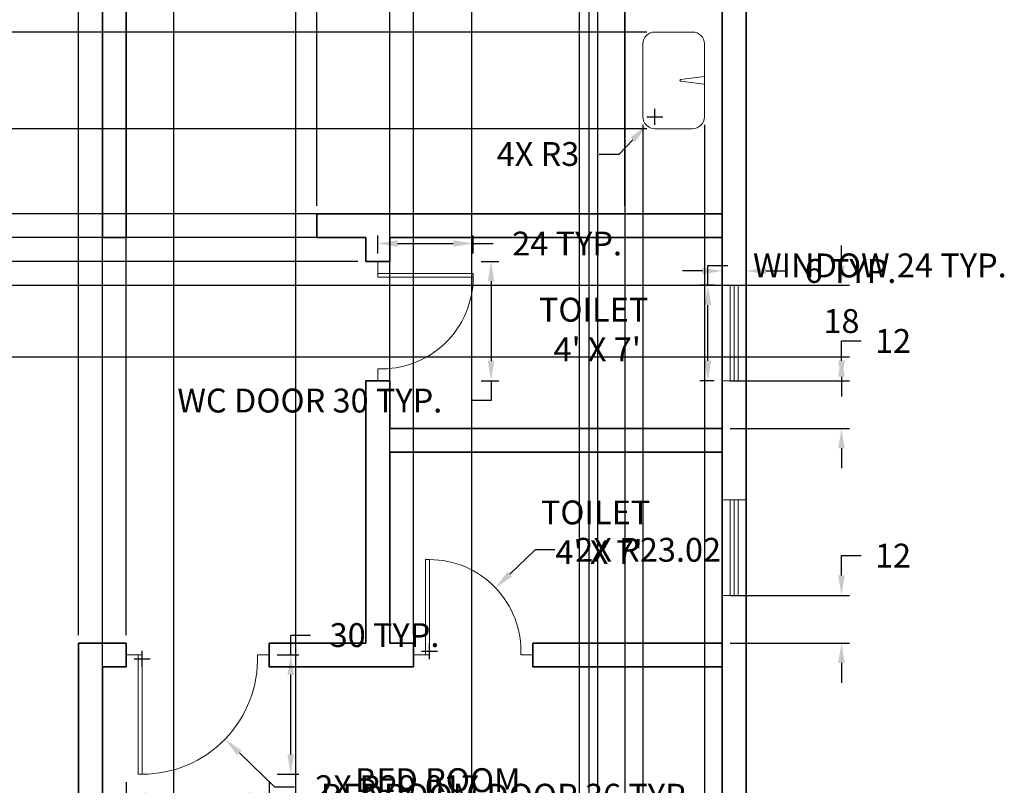
# Model space of a CAD drawing. Units: inches. Extents: x 185 to 668, y 153 to 689.
# Tile 4 of 5: x 420 to 668, y 380 to 572. Entities that reach past the tile are written whole.
import ezdxf

# ---------------------------------------------------------------- set-up
doc = ezdxf.new("R2010")
doc.units = ezdxf.units.IN
doc.header["$MEASUREMENT"] = 0
for name, color, linetype, lineweight in [('A-ANNO-DIMS', 2, 'Continuous', 18), ('A-AREA-IDEN', 7, 'Continuous', 25), ('A-DOOR', 3, 'Continuous', 18), ('A-FLOR-CASE', 8, 'Continuous', 25), ('A-FLOR-FIXT', 9, 'Continuous', 18), ('A-GLAZ', 4, 'Continuous', 18), ('A-WALL', 7, 'Continuous', 35)]:
    doc.layers.add(name, color=color, linetype=linetype, lineweight=lineweight)
doc.styles.get("Standard").update_dxf_attribs({"font": 'arial.ttf'})
doc.dimstyles.get("Standard").update_dxf_attribs({"dimtxt": 6, "dimasz": 5, "dimexe": 2, "dimexo": 2, "dimgap": 4, "dimtad": 0, "dimtih": 1, "dimtoh": 1, "dimdec": 0, "dimzin": 0, "dimdsep": 46, "dimlunit": 3, "dimtxsty": 'Standard', "dimcen": 2, "dimadec": 0, "dimazin": 0, "dimtfac": 1, "dimtdec": 0, "dimtofl": 0, "dimtmove": 0, "dimatfit": 3, "dimfxl": 1, "dimtolj": 1, "dimtzin": 0, "dimarcsym": 0})

# ---------------------------------------------------------------- blocks, each defined once
blk = doc.blocks.new('WINDOW-24')
for p, q in [((2, 24), (0, 24)), ((4, 24), (2, 24)), ((2, 24), (2, 0)), ((3, 24), (3, 0)), ((4, 0), (4, 24)), ((4, 24), (6, 24)), ((2, 0), (0, 0)), ((2, 0), (4, 0)), ((4, 0), (6, 0))]:
    blk.add_line(p, q)
blk = doc.blocks.new('DOOR-SINGLE-30')
for p, q in [((3, 30), (0, 30)), ((3, 30), (3, 0)), ((4, 30), (3, 30)), ((4, 0), (4, 30)), ((33, 30), (36, 30)), ((3, 0), (4, 0))]:
    blk.add_line(p, q)
blk.add_arc((4, 29.02), 29.02, 270, 1.942)
blk = doc.blocks.new('DOOR-SINGLE-24')
for p, q in [((3, 0), (3, 24)), ((3, 24), (4, 24)), ((4, 24), (4, 0)), ((0, 0), (3, 0)), ((4, 0), (3, 0)), ((27, 0), (30, 0))]:
    blk.add_line(p, q)
blk.add_arc((4, 0.98), 23.02, 357.5622, 90)
blk = doc.blocks.new('*D19')
at = {"layer": 'A-ANNO-DIMS', "color": 0, "lineweight": -2, "transparency": 16777216}
for p, q in [((593.44, 505.38), (593.44, 510.38)), ((593.44, 510.38), (598.44, 510.38)), ((595.04, 505.38), (591.44, 505.38)), ((593.44, 486.38), (593.44, 500.38)), ((595.04, 481.38), (591.44, 481.38))]:
    blk.add_line(p, q, dxfattribs=at)
at = {"layer": 'A-ANNO-DIMS', "color": 0, "transparency": 16777216}
for points in [[(592.61, 500.38), (594.27, 500.38), (593.44, 505.38)], [(592.61, 486.38), (594.27, 486.38), (593.44, 481.38)]]:
    blk.add_solid(points, dxfattribs=at)
at = {"layer": 'Defpoints', "color": 0, "transparency": 16777216}
for p in [(593.44, 505.38), (597.04, 505.38), (597.04, 481.38)]:
    blk.add_point(p, dxfattribs=at)
at = {"layer": 'A-ANNO-DIMS', "color": 0, "transparency": 16777216, "insert": (636.72, 510.38), "char_height": 6, "attachment_point": 5}
blk.add_mtext('\\A1;WINDOW 24 TYP.', dxfattribs=at)
blk = doc.blocks.new('*D20')
at = {"layer": 'A-ANNO-DIMS', "color": 0, "lineweight": -2, "transparency": 16777216}
for p, q in [((597.04, 507.38), (597.04, 510.98)), ((603.04, 507.38), (603.04, 510.98)), ((592.04, 508.98), (587.04, 508.98)), ((608.04, 508.98), (613.04, 508.98))]:
    blk.add_line(p, q, dxfattribs=at)
at = {"layer": 'A-ANNO-DIMS', "color": 0, "transparency": 16777216}
for points in [[(592.04, 509.81), (592.04, 508.15), (597.04, 508.98)], [(608.04, 509.81), (608.04, 508.15), (603.04, 508.98)]]:
    blk.add_solid(points, dxfattribs=at)
at = {"layer": 'Defpoints', "color": 0, "transparency": 16777216}
for p in [(603.04, 508.98), (597.04, 505.38), (603.04, 505.38)]:
    blk.add_point(p, dxfattribs=at)
at = {"layer": 'A-ANNO-DIMS', "color": 0, "transparency": 16777216, "insert": (629.33, 508.98), "char_height": 6, "attachment_point": 5}
blk.add_mtext('\\A1;6 TYP.', dxfattribs=at)
blk = doc.blocks.new('*D21')
at = {"layer": 'A-ANNO-DIMS', "color": 0, "lineweight": -2, "transparency": 16777216}
for p, q in [((447.04, 380.38), (447.04, 374.98)), ((483.04, 380.38), (483.04, 374.98)), ((452.04, 376.98), (478.04, 376.98)), ((483.04, 376.98), (488.04, 376.98))]:
    blk.add_line(p, q, dxfattribs=at)
at = {"layer": 'A-ANNO-DIMS', "color": 0, "transparency": 16777216}
for points in [[(452.04, 377.81), (452.04, 376.15), (447.04, 376.98)], [(478.04, 377.81), (478.04, 376.15), (483.04, 376.98)]]:
    blk.add_solid(points, dxfattribs=at)
at = {"layer": 'Defpoints', "color": 0, "transparency": 16777216}
for p in [(447.04, 382.38), (483.04, 382.38), (483.04, 376.98)]:
    blk.add_point(p, dxfattribs=at)
at = {"layer": 'A-ANNO-DIMS', "color": 0, "transparency": 16777216, "insert": (543.07, 376.98), "char_height": 6, "attachment_point": 5}
blk.add_mtext('\\A1;BEDROOM DOOR 36 TYP.', dxfattribs=at)
blk = doc.blocks.new('*D22')
at = {"layer": 'A-ANNO-DIMS', "color": 0, "lineweight": -2, "transparency": 16777216}
for p, q in [((488.44, 412.38), (488.44, 417.38)), ((488.44, 417.38), (493.44, 417.38)), ((485.04, 412.38), (490.44, 412.38)), ((488.44, 387.38), (488.44, 407.38)), ((485.04, 382.38), (490.44, 382.38))]:
    blk.add_line(p, q, dxfattribs=at)
at = {"layer": 'A-ANNO-DIMS', "color": 0, "transparency": 16777216}
for points in [[(487.61, 407.38), (489.27, 407.38), (488.44, 412.38)], [(487.61, 387.38), (489.27, 387.38), (488.44, 382.38)]]:
    blk.add_solid(points, dxfattribs=at)
at = {"layer": 'Defpoints', "color": 0, "transparency": 16777216}
for p in [(483.04, 412.38), (488.44, 412.38), (483.04, 382.38)]:
    blk.add_point(p, dxfattribs=at)
at = {"layer": 'A-ANNO-DIMS', "color": 0, "transparency": 16777216, "insert": (512.04, 417.38), "char_height": 6, "attachment_point": 5}
blk.add_mtext('\\A1;30 TYP.', dxfattribs=at)
blk = doc.blocks.new('*D23')
at = {"layer": 'A-ANNO-DIMS', "color": 0, "lineweight": -2, "transparency": 16777216}
for p, q in [((536.35, 511.38), (540.85, 511.38)), ((538.85, 506.38), (538.85, 486.38)), ((536.35, 481.38), (540.85, 481.38)), ((538.85, 481.38), (538.85, 476.38)), ((538.85, 476.38), (533.85, 476.38))]:
    blk.add_line(p, q, dxfattribs=at)
at = {"layer": 'A-ANNO-DIMS', "color": 0, "transparency": 16777216}
for points in [[(538.02, 506.38), (539.68, 506.38), (538.85, 511.38)], [(538.02, 486.38), (539.68, 486.38), (538.85, 481.38)]]:
    blk.add_solid(points, dxfattribs=at)
at = {"layer": 'Defpoints', "color": 0, "transparency": 16777216}
for p in [(534.35, 511.38), (534.35, 481.38), (538.85, 481.38)]:
    blk.add_point(p, dxfattribs=at)
at = {"layer": 'A-ANNO-DIMS', "color": 0, "transparency": 16777216, "insert": (493.24, 476.38), "char_height": 6, "attachment_point": 5}
blk.add_mtext('\\A1;WC DOOR 30 TYP.', dxfattribs=at)
blk = doc.blocks.new('*D24')
at = {"layer": 'A-ANNO-DIMS', "color": 0, "lineweight": -2, "transparency": 16777216}
for p, q in [((510.35, 513.38), (510.35, 517.88)), ((515.35, 515.88), (529.35, 515.88)), ((534.35, 513.38), (534.35, 517.88)), ((534.35, 515.88), (539.35, 515.88))]:
    blk.add_line(p, q, dxfattribs=at)
at = {"layer": 'A-ANNO-DIMS', "color": 0, "transparency": 16777216}
for points in [[(515.35, 516.71), (515.35, 515.05), (510.35, 515.88)], [(529.35, 516.71), (529.35, 515.05), (534.35, 515.88)]]:
    blk.add_solid(points, dxfattribs=at)
at = {"layer": 'Defpoints', "color": 0, "transparency": 16777216}
for p in [(534.35, 515.88), (510.35, 511.38), (534.35, 511.38)]:
    blk.add_point(p, dxfattribs=at)
at = {"layer": 'A-ANNO-DIMS', "color": 0, "transparency": 16777216, "insert": (558, 515.88), "char_height": 6, "attachment_point": 5}
blk.add_mtext('\\A1;24 TYP.', dxfattribs=at)
blk = doc.blocks.new('*D33')
at = {"layer": 'A-ANNO-DIMS', "color": 0, "lineweight": -2, "transparency": 16777216}
for p, q in [((565.69, 653.38), (565.69, 155.36)), ((597.04, 653.38), (597.04, 155.36)), ((560.69, 157.36), (555.69, 157.36)), ((602.04, 157.36), (607.04, 157.36))]:
    blk.add_line(p, q, dxfattribs=at)
at = {"layer": 'A-ANNO-DIMS', "color": 0, "transparency": 16777216}
for points in [[(560.69, 158.19), (560.69, 156.53), (565.69, 157.36)], [(602.04, 158.19), (602.04, 156.53), (597.04, 157.36)]]:
    blk.add_solid(points, dxfattribs=at)
at = {"layer": 'Defpoints', "color": 0, "transparency": 16777216}
for p in [(565.69, 655.38), (597.04, 655.38), (597.04, 157.36)]:
    blk.add_point(p, dxfattribs=at)
at = {"layer": 'A-ANNO-DIMS', "color": 0, "transparency": 16777216, "insert": (581.37, 157.36), "char_height": 6, "attachment_point": 5}
blk.add_mtext('\\A1;31.35', dxfattribs=at)
blk = doc.blocks.new('*D37')
at = {"layer": 'A-ANNO-DIMS', "color": 0, "lineweight": -2, "transparency": 16777216}
for p, q in [((627.06, 432.38), (627.06, 437.38)), ((627.06, 437.38), (632.06, 437.38)), ((599.04, 427.38), (629.06, 427.38)), ((599.04, 415.38), (629.06, 415.38)), ((627.06, 410.38), (627.06, 405.38))]:
    blk.add_line(p, q, dxfattribs=at)
at = {"layer": 'A-ANNO-DIMS', "color": 0, "transparency": 16777216}
for points in [[(626.23, 432.38), (627.89, 432.38), (627.06, 427.38)], [(626.23, 410.38), (627.89, 410.38), (627.06, 415.38)]]:
    blk.add_solid(points, dxfattribs=at)
at = {"layer": 'Defpoints', "color": 0, "transparency": 16777216}
for p in [(597.04, 427.38), (627.06, 427.38), (597.04, 415.38)]:
    blk.add_point(p, dxfattribs=at)
at = {"layer": 'A-ANNO-DIMS', "color": 0, "transparency": 16777216, "insert": (640.04, 437.38), "char_height": 6, "attachment_point": 5}
blk.add_mtext('\\A1;12', dxfattribs=at)
blk = doc.blocks.new('*D38')
at = {"layer": 'A-ANNO-DIMS', "color": 0, "lineweight": -2, "transparency": 16777216}
for p, q in [((627.06, 486.38), (627.06, 491.38)), ((627.06, 491.38), (632.06, 491.38)), ((599.04, 481.38), (629.06, 481.38)), ((599.04, 469.38), (629.06, 469.38)), ((627.06, 464.38), (627.06, 459.38))]:
    blk.add_line(p, q, dxfattribs=at)
at = {"layer": 'A-ANNO-DIMS', "color": 0, "transparency": 16777216}
for points in [[(626.23, 486.38), (627.89, 486.38), (627.06, 481.38)], [(626.23, 464.38), (627.89, 464.38), (627.06, 469.38)]]:
    blk.add_solid(points, dxfattribs=at)
at = {"layer": 'Defpoints', "color": 0, "transparency": 16777216}
for p in [(597.04, 481.38), (627.06, 481.38), (597.04, 469.38)]:
    blk.add_point(p, dxfattribs=at)
at = {"layer": 'A-ANNO-DIMS', "color": 0, "transparency": 16777216, "insert": (640.04, 491.38), "char_height": 6, "attachment_point": 5}
blk.add_mtext('\\A1;12', dxfattribs=at)
blk = doc.blocks.new('*D43')
at = {"layer": 'A-ANNO-DIMS', "color": 0, "lineweight": -2, "transparency": 16777216}
for p, q in [((489.63, 629.38), (489.63, 155.36)), ((572.5, 629.38), (572.5, 155.36)), ((494.63, 157.36), (516.94, 157.36)), ((567.5, 157.36), (545.19, 157.36))]:
    blk.add_line(p, q, dxfattribs=at)
at = {"layer": 'A-ANNO-DIMS', "color": 0, "transparency": 16777216}
for points in [[(494.63, 158.19), (494.63, 156.53), (489.63, 157.36)], [(567.5, 158.19), (567.5, 156.53), (572.5, 157.36)]]:
    blk.add_solid(points, dxfattribs=at)
at = {"layer": 'Defpoints', "color": 0, "transparency": 16777216}
for p in [(489.63, 631.38), (572.5, 631.38), (572.5, 157.36)]:
    blk.add_point(p, dxfattribs=at)
at = {"layer": 'A-ANNO-DIMS', "color": 0, "transparency": 16777216, "insert": (531.06, 157.36), "char_height": 6, "attachment_point": 5}
blk.add_mtext('\\A1;82.86', dxfattribs=at)
blk = doc.blocks.new('*D44')
at = {"layer": 'A-ANNO-DIMS', "color": 0, "lineweight": -2, "transparency": 16777216}
for p, q in [((447.04, 519.38), (447.04, 687.4)), ((495.04, 525.38), (495.04, 687.4)), ((452.04, 685.4), (462.62, 685.4)), ((490.04, 685.4), (479.47, 685.4))]:
    blk.add_line(p, q, dxfattribs=at)
at = {"layer": 'A-ANNO-DIMS', "color": 0, "transparency": 16777216}
for points in [[(452.04, 686.23), (452.04, 684.56), (447.04, 685.4)], [(490.04, 686.23), (490.04, 684.56), (495.04, 685.4)]]:
    blk.add_solid(points, dxfattribs=at)
at = {"layer": 'Defpoints', "color": 0, "transparency": 16777216}
for p in [(495.04, 685.4), (495.04, 523.38), (447.04, 517.38)]:
    blk.add_point(p, dxfattribs=at)
at = {"layer": 'A-ANNO-DIMS', "color": 0, "transparency": 16777216, "insert": (471.04, 685.4), "char_height": 6, "attachment_point": 5}
blk.add_mtext('\\A1;48', dxfattribs=at)
blk = doc.blocks.new('*D45')
at = {"layer": 'A-ANNO-DIMS', "color": 0, "lineweight": -2, "transparency": 16777216}
for p, q in [((435.04, 417.38), (435.04, 687.4)), ((447.04, 417.38), (447.04, 687.4)), ((430.04, 685.4), (425.04, 685.4)), ((452.04, 685.4), (457.04, 685.4))]:
    blk.add_line(p, q, dxfattribs=at)
at = {"layer": 'A-ANNO-DIMS', "color": 0, "transparency": 16777216}
for points in [[(430.04, 686.23), (430.04, 684.56), (435.04, 685.4)], [(452.04, 686.23), (452.04, 684.56), (447.04, 685.4)]]:
    blk.add_solid(points, dxfattribs=at)
at = {"layer": 'Defpoints', "color": 0, "transparency": 16777216}
for p in [(447.04, 685.4), (435.04, 415.38), (447.04, 415.38)]:
    blk.add_point(p, dxfattribs=at)
at = {"layer": 'A-ANNO-DIMS', "color": 0, "transparency": 16777216, "insert": (465.03, 685.4), "char_height": 6, "attachment_point": 5}
blk.add_mtext('\\A1;12', dxfattribs=at)
blk = doc.blocks.new('*D46')
at = {"layer": 'A-ANNO-DIMS', "color": 0, "lineweight": -2, "transparency": 16777216}
for p, q in [((513.35, 417.38), (513.35, 687.4)), ((519.35, 417.38), (519.35, 687.4)), ((508.35, 685.4), (503.35, 685.4)), ((524.35, 685.4), (529.35, 685.4))]:
    blk.add_line(p, q, dxfattribs=at)
at = {"layer": 'A-ANNO-DIMS', "color": 0, "transparency": 16777216}
for points in [[(508.35, 686.23), (508.35, 684.56), (513.35, 685.4)], [(524.35, 686.23), (524.35, 684.56), (519.35, 685.4)]]:
    blk.add_solid(points, dxfattribs=at)
at = {"layer": 'Defpoints', "color": 0, "transparency": 16777216}
for p in [(519.35, 685.4), (513.35, 415.38), (519.35, 415.38)]:
    blk.add_point(p, dxfattribs=at)
at = {"layer": 'A-ANNO-DIMS', "color": 0, "transparency": 16777216, "insert": (535.33, 685.4), "char_height": 6, "attachment_point": 5}
blk.add_mtext('\\A1;6', dxfattribs=at)
blk = doc.blocks.new('*D47')
at = {"layer": 'A-ANNO-DIMS', "color": 0, "lineweight": -2, "transparency": 16777216}
for p, q in [((219.02, 522.38), (219.02, 527.38)), ((219.02, 527.38), (224.02, 527.38)), ((505.35, 517.38), (217.02, 517.38)), ((505.35, 511.38), (217.02, 511.38)), ((219.02, 506.38), (219.02, 501.38))]:
    blk.add_line(p, q, dxfattribs=at)
at = {"layer": 'A-ANNO-DIMS', "color": 0, "transparency": 16777216}
for points in [[(218.19, 522.38), (219.86, 522.38), (219.02, 517.38)], [(218.19, 506.38), (219.86, 506.38), (219.02, 511.38)]]:
    blk.add_solid(points, dxfattribs=at)
at = {"layer": 'Defpoints', "color": 0, "transparency": 16777216}
for p in [(219.02, 517.38), (507.35, 517.38), (507.35, 511.38)]:
    blk.add_point(p, dxfattribs=at)
at = {"layer": 'A-ANNO-DIMS', "color": 0, "transparency": 16777216, "insert": (230, 527.38), "char_height": 6, "attachment_point": 5}
blk.add_mtext('\\A1;6', dxfattribs=at)
blk = doc.blocks.new('*D49')
at = {"layer": 'A-ANNO-DIMS', "color": 0, "lineweight": -2, "transparency": 16777216}
for p, q in [((572.5, 525.38), (572.5, 687.4)), ((597.04, 525.38), (597.04, 687.4)), ((577.5, 685.4), (592.04, 685.4)), ((597.04, 685.4), (602.04, 685.4))]:
    blk.add_line(p, q, dxfattribs=at)
at = {"layer": 'A-ANNO-DIMS', "color": 0, "transparency": 16777216}
for points in [[(577.5, 686.23), (577.5, 684.56), (572.5, 685.4)], [(592.04, 686.23), (592.04, 684.56), (597.04, 685.4)]]:
    blk.add_solid(points, dxfattribs=at)
at = {"layer": 'Defpoints', "color": 0, "transparency": 16777216}
for p in [(597.04, 685.4), (572.5, 523.38), (597.04, 523.38)]:
    blk.add_point(p, dxfattribs=at)
at = {"layer": 'A-ANNO-DIMS', "color": 0, "transparency": 16777216, "insert": (618.54, 685.4), "char_height": 6, "attachment_point": 5}
blk.add_mtext('\\A1;24.546', dxfattribs=at)
blk = doc.blocks.new('*D51')
at = {"layer": 'A-ANNO-DIMS', "color": 0, "lineweight": -2, "transparency": 16777216}
for p, q in [((627.06, 510.38), (627.06, 515.38)), ((329.04, 505.38), (629.06, 505.38)), ((329.04, 487.38), (629.06, 487.38)), ((627.06, 482.38), (627.06, 477.38))]:
    blk.add_line(p, q, dxfattribs=at)
at = {"layer": 'A-ANNO-DIMS', "color": 0, "transparency": 16777216}
for points in [[(626.23, 510.38), (627.89, 510.38), (627.06, 505.38)], [(626.23, 482.38), (627.89, 482.38), (627.06, 487.38)]]:
    blk.add_solid(points, dxfattribs=at)
at = {"layer": 'Defpoints', "color": 0, "transparency": 16777216}
for p in [(327.04, 505.38), (627.06, 505.38), (327.04, 487.38)]:
    blk.add_point(p, dxfattribs=at)
at = {"layer": 'A-ANNO-DIMS', "color": 0, "transparency": 16777216, "insert": (627.06, 496.38), "char_height": 6, "attachment_point": 5}
blk.add_mtext('\\A1;18', dxfattribs=at)
blk = doc.blocks.new('*D52')
at = {"layer": 'A-ANNO-DIMS', "color": 0, "lineweight": -2, "transparency": 16777216}
for p, q in [((441.04, 344.34), (441.04, 687.4)), ((459.04, 344.34), (459.04, 687.4)), ((436.04, 685.4), (431.04, 685.4)), ((464.04, 685.4), (469.04, 685.4))]:
    blk.add_line(p, q, dxfattribs=at)
at = {"layer": 'A-ANNO-DIMS', "color": 0, "transparency": 16777216}
for points in [[(436.04, 686.23), (436.04, 684.56), (441.04, 685.4)], [(464.04, 686.23), (464.04, 684.56), (459.04, 685.4)]]:
    blk.add_solid(points, dxfattribs=at)
at = {"layer": 'Defpoints', "color": 0, "transparency": 16777216}
for p in [(459.04, 685.4), (441.04, 342.34), (459.04, 342.34)]:
    blk.add_point(p, dxfattribs=at)
at = {"layer": 'A-ANNO-DIMS', "color": 0, "transparency": 16777216, "insert": (450.04, 685.4), "char_height": 6, "attachment_point": 5}
blk.add_mtext('\\A1;18', dxfattribs=at)
blk = doc.blocks.new('*D62')
at = {"layer": 'A-ANNO-DIMS', "color": 0, "lineweight": -2, "transparency": 16777216}
for p, q in [((533.97, 632.47), (533.97, 155.36)), ((563.51, 632.47), (563.51, 155.36)), ((538.97, 157.36), (558.51, 157.36)), ((563.51, 157.36), (568.51, 157.36))]:
    blk.add_line(p, q, dxfattribs=at)
at = {"layer": 'A-ANNO-DIMS', "color": 0, "transparency": 16777216}
for points in [[(538.97, 158.19), (538.97, 156.53), (533.97, 157.36)], [(558.51, 158.19), (558.51, 156.53), (563.51, 157.36)]]:
    blk.add_solid(points, dxfattribs=at)
at = {"layer": 'Defpoints', "color": 0, "transparency": 16777216}
for p in [(533.97, 634.47), (563.51, 634.47), (563.51, 157.36)]:
    blk.add_point(p, dxfattribs=at)
at = {"layer": 'A-ANNO-DIMS', "color": 0, "transparency": 16777216, "insert": (585.01, 157.36), "char_height": 6, "attachment_point": 5}
blk.add_mtext('\\A1;29.536', dxfattribs=at)
blk = doc.blocks.new('*D65')
at = {"layer": 'A-ANNO-DIMS', "color": 0, "lineweight": -2, "transparency": 16777216}
for p, q in [((577.09, 545.77), (577.09, 155.36)), ((592.55, 545.77), (592.55, 155.36)), ((572.09, 157.36), (567.09, 157.36)), ((597.55, 157.36), (602.55, 157.36))]:
    blk.add_line(p, q, dxfattribs=at)
at = {"layer": 'A-ANNO-DIMS', "color": 0, "transparency": 16777216}
for points in [[(572.09, 158.19), (572.09, 156.53), (577.09, 157.36)], [(597.55, 158.19), (597.55, 156.53), (592.55, 157.36)]]:
    blk.add_solid(points, dxfattribs=at)
at = {"layer": 'Defpoints', "color": 0, "transparency": 16777216}
for p in [(577.09, 547.77), (592.55, 547.77), (592.55, 157.36)]:
    blk.add_point(p, dxfattribs=at)
at = {"layer": 'A-ANNO-DIMS', "color": 0, "transparency": 16777216, "insert": (618.73, 157.36), "char_height": 6, "attachment_point": 5}
blk.add_mtext('\\A1;15.467', dxfattribs=at)
blk = doc.blocks.new('*D66')
at = {"layer": 'A-ANNO-DIMS', "color": 0, "lineweight": -2, "transparency": 16777216}
for p, q in [((219.02, 569.09), (219.02, 574.09)), ((219.02, 574.09), (224.02, 574.09)), ((578.09, 569.09), (217.02, 569.09)), ((219.02, 549.77), (219.02, 564.09)), ((578.09, 544.77), (217.02, 544.77))]:
    blk.add_line(p, q, dxfattribs=at)
at = {"layer": 'A-ANNO-DIMS', "color": 0, "transparency": 16777216}
for points in [[(218.19, 564.09), (219.86, 564.09), (219.02, 569.09)], [(218.19, 549.77), (219.86, 549.77), (219.02, 544.77)]]:
    blk.add_solid(points, dxfattribs=at)
at = {"layer": 'Defpoints', "color": 0, "transparency": 16777216}
for p in [(219.02, 569.09), (580.09, 569.09), (580.09, 544.77)]:
    blk.add_point(p, dxfattribs=at)
at = {"layer": 'A-ANNO-DIMS', "color": 0, "transparency": 16777216, "insert": (240.55, 574.09), "char_height": 6, "attachment_point": 5}
blk.add_mtext('\\A1;24.315', dxfattribs=at)
blk = doc.blocks.new('*D69')
at = {"layer": 'A-ANNO-DIMS', "color": 0, "lineweight": -2, "transparency": 16777216}
for p, q in [((219.02, 544.77), (219.02, 549.77)), ((219.02, 549.77), (224.02, 549.77)), ((578.09, 544.77), (217.02, 544.77)), ((219.02, 528.38), (219.02, 539.77)), ((570.5, 523.38), (217.02, 523.38))]:
    blk.add_line(p, q, dxfattribs=at)
at = {"layer": 'A-ANNO-DIMS', "color": 0, "transparency": 16777216}
for points in [[(218.19, 539.77), (219.86, 539.77), (219.02, 544.77)], [(218.19, 528.38), (219.86, 528.38), (219.02, 523.38)]]:
    blk.add_solid(points, dxfattribs=at)
at = {"layer": 'Defpoints', "color": 0, "transparency": 16777216}
for p in [(219.02, 544.77), (580.09, 544.77), (572.5, 523.38)]:
    blk.add_point(p, dxfattribs=at)
at = {"layer": 'A-ANNO-DIMS', "color": 0, "transparency": 16777216, "insert": (238.2, 549.77), "char_height": 6, "attachment_point": 5}
blk.add_mtext('\\A1;21.39', dxfattribs=at)
blk = doc.blocks.new('*D74')
at = {"layer": 'A-ANNO-DIMS', "color": 0, "lineweight": -2, "transparency": 16777216}
for p, q in [((561.08, 272.34), (561.08, 687.4)), ((597.04, 267.38), (597.04, 687.4)), ((556.08, 685.4), (551.08, 685.4)), ((602.04, 685.4), (607.04, 685.4))]:
    blk.add_line(p, q, dxfattribs=at)
at = {"layer": 'A-ANNO-DIMS', "color": 0, "transparency": 16777216}
for points in [[(556.08, 686.23), (556.08, 684.56), (561.08, 685.4)], [(602.04, 686.23), (602.04, 684.56), (597.04, 685.4)]]:
    blk.add_solid(points, dxfattribs=at)
at = {"layer": 'Defpoints', "color": 0, "transparency": 16777216}
for p in [(597.04, 685.4), (561.08, 270.34), (597.04, 265.38)]:
    blk.add_point(p, dxfattribs=at)
at = {"layer": 'A-ANNO-DIMS', "color": 0, "transparency": 16777216, "insert": (579.06, 685.4), "char_height": 6, "attachment_point": 5}
blk.add_mtext('\\A1;35.96', dxfattribs=at)
blk = doc.blocks.new('*D77')
at = {"layer": 'A-ANNO-DIMS', "color": 0, "lineweight": -2, "transparency": 16777216}
for p, q in [((451.04, 409.4), (451.04, 413.4)), ((449.04, 411.4), (453.04, 411.4)), ((484.42, 379.13), (475.5, 387.75)), ((489.42, 379.13), (484.42, 379.13))]:
    blk.add_line(p, q, dxfattribs=at)
at = {"layer": 'A-ANNO-DIMS', "color": 0, "transparency": 16777216}
blk.add_solid([(476.08, 388.35), (474.92, 387.15), (471.9, 391.23)], dxfattribs=at)
at = {"layer": 'Defpoints', "color": 0, "transparency": 16777216}
for p in [(451.04, 411.4), (471.9, 391.23)]:
    blk.add_point(p, dxfattribs=at)
at = {"layer": 'A-ANNO-DIMS', "color": 0, "transparency": 16777216, "insert": (515.24, 379.13), "char_height": 6, "attachment_point": 5}
blk.add_mtext('\\A1;2X R29.017', dxfattribs=at)
blk = doc.blocks.new('*D78')
at = {"layer": 'A-ANNO-DIMS', "color": 0, "lineweight": -2, "transparency": 16777216}
for p, q in [((549.94, 438.84), (543.58, 432.75)), ((554.94, 438.84), (549.94, 438.84)), ((523.35, 411.36), (523.35, 415.36)), ((521.35, 413.36), (525.35, 413.36))]:
    blk.add_line(p, q, dxfattribs=at)
at = {"layer": 'A-ANNO-DIMS', "color": 0, "transparency": 16777216}
blk.add_solid([(543, 433.35), (544.16, 432.14), (539.97, 429.29)], dxfattribs=at)
at = {"layer": 'Defpoints', "color": 0, "transparency": 16777216}
for p in [(539.97, 429.29), (523.35, 413.36)]:
    blk.add_point(p, dxfattribs=at)
at = {"layer": 'A-ANNO-DIMS', "color": 0, "transparency": 16777216, "insert": (578.4, 438.84), "char_height": 6, "attachment_point": 5}
blk.add_mtext('\\A1;2X R23.02', dxfattribs=at)
blk = doc.blocks.new('*D80')
at = {"layer": 'A-ANNO-DIMS', "color": 0, "lineweight": -2, "transparency": 16777216}
for p, q in [((578.09, 547.77), (582.09, 547.77)), ((580.09, 545.77), (580.09, 549.77)), ((571.08, 538.4), (574.54, 542)), ((566.08, 538.4), (571.08, 538.4))]:
    blk.add_line(p, q, dxfattribs=at)
at = {"layer": 'A-ANNO-DIMS', "color": 0, "transparency": 16777216}
blk.add_solid([(573.94, 542.58), (575.14, 541.43), (578.01, 545.61)], dxfattribs=at)
at = {"layer": 'Defpoints', "color": 0, "transparency": 16777216}
for p in [(580.09, 547.77), (578.01, 545.61)]:
    blk.add_point(p, dxfattribs=at)
at = {"layer": 'A-ANNO-DIMS', "color": 0, "transparency": 16777216, "insert": (550.67, 538.4), "char_height": 6, "attachment_point": 5}
blk.add_mtext('\\A1;4X R3', dxfattribs=at)

msp = doc.modelspace()

# ---------------------------------------------------------------- linework, layer by layer
at = {"layer": 'A-FLOR-CASE'}
msp.add_line((572.4952, 631.3789), (572.4952, 523.3789), dxfattribs=at)
at = {"layer": 'A-FLOR-FIXT'}
for p, q in [((592.5536, 557.9326), (586.503, 557.1469)), ((586.503, 556.7108), (592.5536, 555.9284))]:
    msp.add_line(p, q, dxfattribs=at)
msp.add_lwpolyline([(577.0867, 566.0859, -0.41421356), (580.0867, 569.0859), (589.5536, 569.0859, -0.41421356), (592.5536, 566.0859), (592.5536, 547.7709, -0.41421356), (589.5536, 544.7709), (580.0867, 544.7709, -0.41421356), (577.0867, 547.7709)], format="xyb", close=True, dxfattribs=at)
msp.add_open_spline([(586.503, 556.7108), (586.3589, 556.7294), (586.3589, 557.1282), (586.503, 557.1469)], degree=3, dxfattribs=at)
at = {"layer": 'A-WALL'}
for p, q in [((603.041, 181.3789), (603.041, 661.3789)), ((447.041, 655.3789), (447.041, 523.3789)), ((597.041, 655.3789), (597.041, 523.3789)), ((441.041, 583.3789), (441.041, 517.3789)), ((447.041, 523.3789), (447.041, 517.3789)), ((597.041, 523.3789), (495.041, 523.3789)), ((495.041, 523.3789), (495.041, 517.3789)), ((447.041, 517.3789), (441.041, 517.3789)), ((507.3502, 517.3789), (495.041, 517.3789)), ((507.3502, 517.3789), (507.3502, 511.3789)), ((597.041, 517.3789), (513.3502, 517.3789)), ((513.3502, 517.3789), (513.3502, 511.3789)), ((597.041, 517.3789), (597.041, 469.3789)), ((513.3502, 511.3789), (507.3502, 511.3789)), ((513.3502, 481.3789), (507.3502, 481.3789)), ((507.3502, 481.3789), (507.3502, 415.3789)), ((513.3502, 481.3789), (513.3502, 469.3789)), ((597.041, 469.3789), (513.3502, 469.3789)), ((597.041, 463.3789), (513.3502, 463.3789)), ((513.3502, 463.3789), (513.3502, 415.3789)), ((597.041, 463.3789), (597.041, 415.3789)), ((435.041, 415.3789), (435.041, 265.3789)), ((447.041, 415.3789), (435.041, 415.3789)), ((447.041, 415.3789), (447.041, 409.3789)), ((483.041, 415.3789), (483.041, 409.3789)), ((507.3502, 415.3789), (483.041, 415.3789)), ((519.3502, 415.3789), (513.3502, 415.3789)), ((519.3502, 415.3789), (519.3502, 409.3789)), ((597.041, 415.3789), (549.3502, 415.3789)), ((549.3502, 415.3789), (549.3502, 409.3789)), ((441.041, 265.3789), (441.041, 409.3789)), ((447.041, 409.3789), (441.041, 409.3789)), ((519.3502, 409.3789), (483.041, 409.3789)), ((597.041, 409.3789), (549.3502, 409.3789)), ((597.041, 409.3789), (597.041, 265.3789))]:
    msp.add_line(p, q, dxfattribs=at)

# ---------------------------------------------------------------- block references
at = {"layer": 'A-DOOR', "rotation": 270.0000000000002}
msp.add_blockref('DOOR-SINGLE-24', (510.3503, 511.3792), dxfattribs=at)
at = {"layer": 'A-DOOR'}
for name, p in [('DOOR-SINGLE-24', (519.35, 412.379)), ('DOOR-SINGLE-30', (447.041, 382.379))]:
    msp.add_blockref(name, p, dxfattribs=at)
at = {"layer": 'A-GLAZ'}
for p in [(597.041, 481.379), (597.041, 427.379)]:
    msp.add_blockref('WINDOW-24', p, dxfattribs=at)

# ---------------------------------------------------------------- texts
at = {"layer": 'A-AREA-IDEN', "char_height": 6, "attachment_point": 1}
for s, insert in [("TOILET\\P  4' X 7'", (550.9107, 502.2462)), ("TOILET\\P  4' X 7'", (551.395, 451.2397)), ("BED ROOM\\P   12' X 13'", (504.606, 383.8904))]:
    msp.add_mtext_dynamic_manual_height_columns(s, width=69.605686, gutter_width=1, heights=[0], dxfattribs=dict(at, insert=insert))

# ---------------------------------------------------------------- dimensions: what is measured, and where the dimension line sits
at = {"layer": 'A-ANNO-DIMS'}
for base, p1, p2, override, picture, middle in [((447.041, 685.3964), (435.041, 415.3789), (447.041, 415.3789), {"dimdec": 0, "dimlfac": 1, "dimrnd": 0, "dimzin": 0, "dimdsep": 46, "dimlunit": 2}, '*D45', (465.0253, 685.3964)), ((459.041, 685.3964), (441.041, 342.3357), (459.041, 342.3357), {"dimdec": 0, "dimlfac": 1, "dimrnd": 0, "dimzin": 0, "dimdsep": 46, "dimlunit": 2}, '*D52', (450.041, 685.3964)), ((495.041, 685.3964), (447.041, 517.3789), (495.041, 523.3789), {"dimdec": 0, "dimlfac": 1, "dimrnd": 0, "dimzin": 0, "dimdsep": 46, "dimlunit": 2}, '*D44', (471.041, 685.3964)), ((519.3502, 685.3964), (513.3502, 415.3789), (519.3502, 415.3789), {"dimdec": 0, "dimlfac": 1, "dimrnd": 0, "dimzin": 0, "dimdsep": 46, "dimlunit": 2}, '*D46', (535.3311, 685.3964)), ((597.041, 685.3964), (561.0793, 270.3357), (597.041, 265.3789), {"dimdec": 2, "dimlfac": 1, "dimrnd": 0, "dimzin": 0, "dimdsep": 46, "dimlunit": 2}, '*D74', (579.0601, 685.3964)), ((597.041, 685.3964), (572.4952, 523.3789), (597.041, 523.3789), {"dimdec": 3, "dimlfac": 1, "dimrnd": 0, "dimzin": 0, "dimdsep": 46, "dimlunit": 2}, '*D49', (618.5444, 685.3964)), ((597.041, 157.3614), (565.6925, 655.3789), (597.041, 655.3789), {"dimdec": 2, "dimlfac": 1, "dimrnd": 0, "dimzin": 0, "dimdsep": 46, "dimlunit": 2}, '*D33', (581.3667, 157.3614)), ((563.5058, 157.3614), (533.9695, 634.4736), (563.5058, 634.4736), {"dimdec": 3, "dimlfac": 1, "dimrnd": 0, "dimzin": 0, "dimdsep": 46, "dimlunit": 2}, '*D62', (585.0092, 157.3614)), ((572.4952, 157.3614), (489.6328, 631.3789), (572.4952, 631.3789), {"dimdec": 2, "dimlfac": 1, "dimrnd": 0, "dimzin": 0, "dimdsep": 46, "dimlunit": 2}, '*D43', (531.064, 157.3614)), ((592.5536, 157.3614), (577.0867, 547.7709), (592.5536, 547.7709), {"dimdec": 3, "dimlfac": 1, "dimrnd": 0, "dimzin": 0, "dimdsep": 46, "dimlunit": 2}, '*D65', (618.7255, 157.3614))]:
    dim = msp.add_linear_dim(base=base, p1=p1, p2=p2, dimstyle='Standard', override=override, dxfattribs=at)
    dim.commit()
    dim.dimension.update_dxf_attribs({"geometry": picture, "text_midpoint": middle})
for base, p1, p2, override, picture, middle in [((219.0235, 569.0859), (580.0867, 544.7709), (580.0867, 569.0859), {"dimdec": 3, "dimlfac": 1, "dimrnd": 0, "dimzin": 0, "dimdsep": 46, "dimlunit": 2}, '*D66', (240.5514, 574.0859)), ((219.0235, 544.7709), (572.4952, 523.3789), (580.0867, 544.7709), {"dimdec": 2, "dimlfac": 1, "dimrnd": 0, "dimzin": 0, "dimdsep": 46, "dimlunit": 2}, '*D69', (238.2042, 549.7709)), ((219.0235, 517.3789), (507.3502, 511.3789), (507.3502, 517.3789), {"dimdec": 0, "dimlfac": 1, "dimrnd": 0, "dimzin": 0, "dimdsep": 46, "dimlunit": 2}, '*D47', (230.0044, 527.3789)), ((627.0585, 505.3789), (327.041, 487.3789), (327.041, 505.3789), {"dimdec": 0, "dimlfac": 1, "dimrnd": 0, "dimzin": 0, "dimdsep": 46, "dimlunit": 2}, '*D51', (627.0585, 496.3789)), ((627.0585, 481.3789), (597.041, 469.3789), (597.041, 481.3789), {"dimdec": 0, "dimlfac": 1, "dimrnd": 0, "dimzin": 0, "dimdsep": 46, "dimlunit": 2}, '*D38', (640.0428, 491.3789)), ((627.0585, 427.3789), (597.041, 415.3789), (597.041, 427.3789), {"dimdec": 0, "dimlfac": 1, "dimrnd": 0, "dimzin": 0, "dimdsep": 46, "dimlunit": 2}, '*D37', (640.0428, 437.3789))]:
    dim = msp.add_linear_dim(base=base, p1=p1, p2=p2, angle=90, dimstyle='Standard', override=override, dxfattribs=at)
    dim.commit()
    dim.dimension.update_dxf_attribs({"geometry": picture, "text_midpoint": middle})
dim = msp.add_radius_dim(center=(580.0867, 547.7709), mpoint=(578.0078, 545.6081), text='4X <>', dimstyle='Standard', override={"dimdec": 0, "dimlfac": 1, "dimrnd": 0, "dimzin": 0, "dimdsep": 46, "dimlunit": 2}, dxfattribs=at)
dim.commit()
dim.dimension.update_dxf_attribs({"geometry": '*D80', "text_midpoint": (550.6733, 538.3986)})
for base, p1, p2, angle, text, picture, middle in [((534.3502, 515.8789), (510.3502, 511.3789), (534.3502, 511.3789), 0, '<> TYP.', '*D24', (558.0044, 515.8789)), ((593.441, 505.3789), (597.041, 481.3789), (597.041, 505.3789), 90, 'WINDOW <> TYP.', '*D19', (636.7199, 510.3789)), ((538.8502, 481.3789), (534.3502, 511.3789), (534.3502, 481.3789), 270, 'WC DOOR <> TYP.', '*D23', (493.2404, 476.3789)), ((488.441, 412.3789), (483.041, 382.3789), (483.041, 412.3789), 90, '<> TYP.', '*D22', (512.0419, 417.3789))]:
    dim = msp.add_linear_dim(base=base, p1=p1, p2=p2, angle=angle, text=text, dimstyle='Standard', override={"dimdec": 0, "dimlfac": 1, "dimrnd": 0, "dimzin": 0, "dimdsep": 46, "dimlunit": 2}, dxfattribs=at)
    dim.commit()
    dim.dimension.update_dxf_attribs({"geometry": picture, "text_midpoint": middle})
for base, p1, p2, text, picture, middle in [((603.041, 508.9789), (597.041, 505.3789), (603.041, 505.3789), '<> TYP.', '*D20', (629.3295, 508.9789)), ((483.041, 376.9789), (447.041, 382.3789), (483.041, 382.3789), 'BEDROOM DOOR <> TYP.', '*D21', (543.0676, 376.9789))]:
    dim = msp.add_linear_dim(base=base, p1=p1, p2=p2, text=text, dimstyle='Standard', override={"dimdec": 0, "dimlfac": 1, "dimrnd": 0, "dimzin": 0, "dimdsep": 46, "dimlunit": 2}, dxfattribs=at)
    dim.commit()
    dim.dimension.update_dxf_attribs({"geometry": picture, "text_midpoint": middle})
for center, mpoint, override, picture, middle in [((523.3502, 413.3581), (539.9712, 429.2862), {"dimdec": 2, "dimlfac": 1, "dimrnd": 0, "dimzin": 0, "dimdsep": 46, "dimlunit": 2}, '*D78', (578.4049, 438.843)), ((451.041, 411.3956), (471.9036, 391.2284), {"dimdec": 3, "dimlfac": 1, "dimrnd": 0, "dimzin": 0, "dimdsep": 46, "dimlunit": 2}, '*D77', (515.2438, 379.128))]:
    dim = msp.add_radius_dim(center=center, mpoint=mpoint, text='2X <>', dimstyle='Standard', override=override, dxfattribs=at)
    dim.commit()
    dim.dimension.update_dxf_attribs({"geometry": picture, "text_midpoint": middle, "dimtype": 164})

doc.saveas('drawing.dxf')
